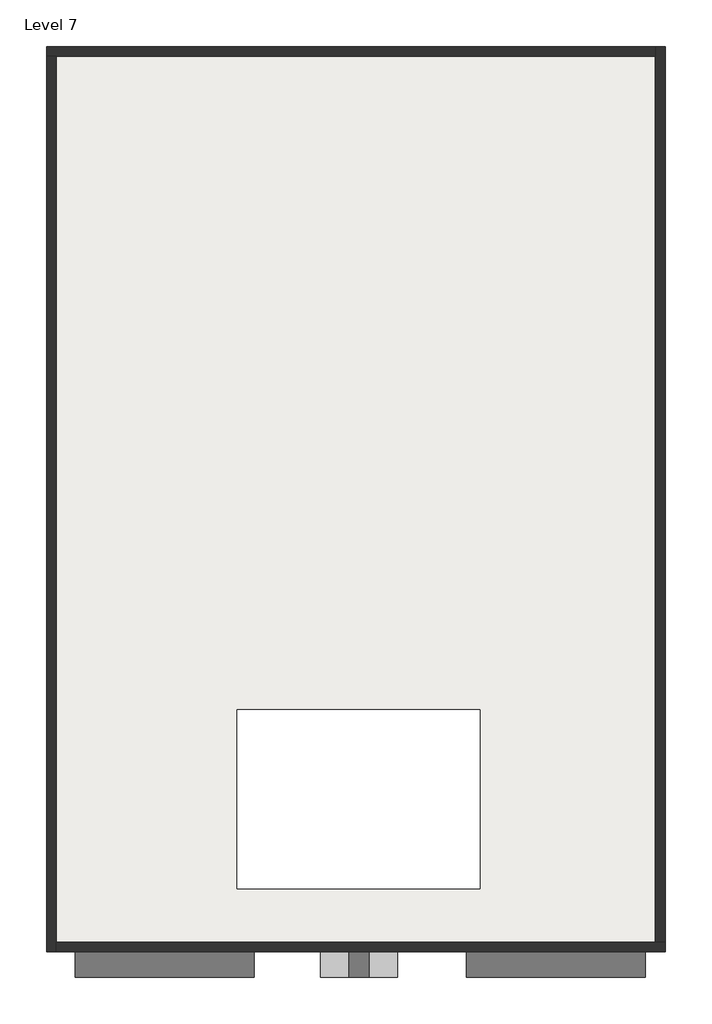
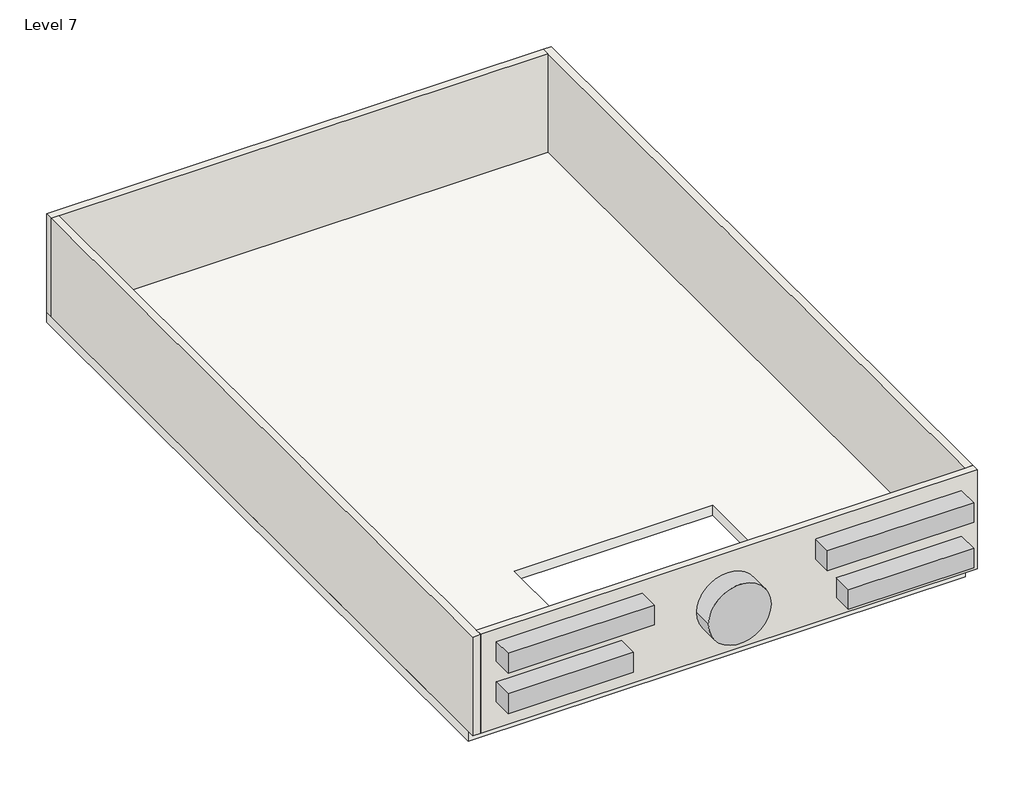
# One storey, incomplete: 4 walls, 1 proxy, 1 roof.
"""IFC4 building model written with IfcOpenShell, lengths in millimetres."""

from ifc_helpers import new_model, si_unit, frame, origin, place, context, project, spatial, polyline, outline, extrude, faceted_brep, transform, mapped, element, save
from components import generic_models_1_generic_models_1_124607eb

model = new_model("IFC4")

# Units and contexts
model_context = context("Model", 3, world=origin())
ifc_project = project(units=[si_unit("LENGTHUNIT", "METRE", prefix="MILLI")], contexts=[model_context])

# Site, building, storey
site = spatial("IfcSite", under=ifc_project)
building = spatial("IfcBuilding", under=site)
storey = spatial("IfcBuildingStorey", under=building, Name="Level 7", Elevation=16002.0)

# Proxy
placement = place(None, origin())
generic_models_1_generic_models_1_shape = generic_models_1_generic_models_1_124607eb(model_context)
element("IfcBuildingElementProxy", 1, Name="Generic Models 1 : Generic Models 1", ObjectType="Generic Models 1 : Generic Models 1", at=placement, inside=storey, context=model_context, shape_type="MappedRepresentation", body=[
    mapped(generic_models_1_generic_models_1_shape, transform((0.0, 0.0, 0.0), x_axis=(1.0, 0.0, 0.0), y_axis=(0.0, 1.0, 0.0), z_axis=(0.0, 0.0, 1.0))),
])

# Roof
element("IfcRoof", 2, ObjectType="Generic - 12\"", at=placement, inside=storey, context=model_context, shape_type="SweptSolid", body=[
    extrude(outline(polyline([(2221.2910386, -5039.0109248), (-5036.7589614, -5039.0109248), (-5036.7589614, 5628.9890752), (2221.2910386, 5628.9890752), (2221.2910386, -5039.0109248)]), holes=[polyline([(131.1896864, -2269.417212), (-2764.4103136, -2269.417212), (-2764.4103136, -4403.017212), (131.1896864, -4403.017212), (131.1896864, -2269.417212)])]), frame((0.0, 0.0, 15849.6), z_axis=(0.0, 0.0, 1.0), x_axis=(1.0, 0.0, 0.0)), (0.0, 0.0, 1.0), 152.4),
])

# Walls
element("IfcWall", 3, ObjectType="4.5\"", at=placement, inside=storey, context=model_context, shape_type="Brep", body=[
    faceted_brep([(-5036.7589614, 5514.6890752, 16002.0), (-4922.4589614, 5514.6890752, 16002.0), (2221.2910386, 5514.6890752, 16002.0), (2221.2910386, 5514.6890752, 17526.0), (-4922.4589614, 5514.6890752, 17526.0), (-5036.7589614, 5514.6890752, 17526.0), (-5036.7589614, 5628.9890752, 16002.0), (-5036.7589614, 5628.9890752, 17526.0), (2221.2910386, 5628.9890752, 17526.0), (2221.2910386, 5628.9890752, 16002.0)], [[[0, 1, 2, 3, 4, 5]], [[6, 7, 8, 9]], [[2, 1, 0, 6, 9]], [[5, 4, 3, 8, 7]], [[0, 5, 7, 6]], [[3, 2, 9, 8]]]),
])
element("IfcWall", 4, ObjectType="4.5\"", at=placement, inside=storey, context=model_context, shape_type="Brep", body=[
    faceted_brep([(-4922.4589614, -5153.3109248, 16002.0), (-4922.4589614, -5039.0109248, 16002.0), (-4922.4589614, 5514.6890752, 16002.0), (-4922.4589614, 5514.6890752, 17526.0), (-4922.4589614, -5039.0109248, 17526.0), (-4922.4589614, -5153.3109248, 17526.0), (-5036.7589614, -5153.3109248, 16002.0), (-5036.7589614, -5153.3109248, 17526.0), (-5036.7589614, 5514.6890752, 17526.0), (-5036.7589614, 5514.6890752, 16002.0)], [[[0, 1, 2, 3, 4, 5]], [[6, 7, 8, 9]], [[2, 1, 0, 6, 9]], [[5, 4, 3, 8, 7]], [[0, 5, 7, 6]], [[3, 2, 9, 8]]]),
])
element("IfcWall", 5, ObjectType="4.5\"", at=placement, inside=storey, context=model_context, shape_type="Brep", body=[
    faceted_brep([(2335.5910386, -5039.0109248, 16002.0), (2221.2910386, -5039.0109248, 16002.0), (-4922.4589614, -5039.0109248, 16002.0), (-4922.4589614, -5039.0109248, 17526.0), (2221.2910386, -5039.0109248, 17526.0), (2335.5910386, -5039.0109248, 17526.0), (2335.5910386, -5153.3109248, 16002.0), (2335.5910386, -5153.3109248, 17526.0), (-4922.4589614, -5153.3109248, 17526.0), (-4922.4589614, -5153.3109248, 16002.0)], [[[0, 1, 2, 3, 4, 5]], [[6, 7, 8, 9]], [[2, 1, 0, 6, 9]], [[5, 4, 3, 8, 7]], [[0, 5, 7, 6]], [[3, 2, 9, 8]]]),
])
element("IfcWall", 6, ObjectType="4.5\"", at=placement, inside=storey, context=model_context, shape_type="Brep", body=[
    faceted_brep([(2221.2910386, 5628.9890752, 16002.0), (2221.2910386, 5514.6890752, 16002.0), (2221.2910386, -5039.0109248, 16002.0), (2221.2910386, -5039.0109248, 17526.0), (2221.2910386, 5514.6890752, 17526.0), (2221.2910386, 5628.9890752, 17526.0), (2335.5910386, 5628.9890752, 16002.0), (2335.5910386, 5628.9890752, 17526.0), (2335.5910386, -5039.0109248, 17526.0), (2335.5910386, -5039.0109248, 16002.0)], [[[0, 1, 2, 3, 4, 5]], [[6, 7, 8, 9]], [[2, 1, 0, 6, 9]], [[5, 4, 3, 8, 7]], [[0, 5, 7, 6]], [[3, 2, 9, 8]]]),
])

save(model, "model.ifc")

# Revit data of these elements
# Type "Generic - 12\""
#   Assembly Code = "B1020"
#   Layers, outside or top first: 0' - 6" no material (function 1)
# Type "4.5\""
#   Assembly Code = "B2010"
#   Layers, outside or top first: 0' - 4 1/2" no material (function 1)
# Element 1 (IfcBuildingElementProxy, "Generic Models 1 : Generic Models 1")
#   Phase Created = New Construction
#   Materials on its faces: "Default Mass Exterior Wall", "Parking Stripe"
# Element 2 (IfcRoof, "Generic - 12\"")
#   built-in parameter 1001705 = 52.5 (stored number, unit not read)
#   built-in parameter 1001701 = -0.5 (stored number, unit not read)
#   built-in parameter 1001710 = 33615
#   Phase Created = New Construction
#   Materials on its faces: "Default Roof", "Door - Frame"
# Elements 3, 4, 5, 6 (IfcWall, "4.5\"")
#   Top Offset = 0' - 0"
#   Base Offset = 0' - 0"
#   Unconnected Height = 5' - 0"
#   wall height = 5' - 0"
#   Phase Created = New Construction
#   Base Constraint = Level 7
#   Materials on its faces: "Default Wall", "Laminate, Ivory, Matte"
# Materials
#   "Default Mass Exterior Wall": class "Generic", colour RGB 133 178 44, transparency 0.2, Cost = 0
#   "Parking Stripe": class "Paint", colour RGB 250 250 91, transparency 0, Cost = 0
#   "Default Roof": colour RGB 88 101 114, transparency 0, Cost = 0
#   "Door - Frame": colour RGB 118 70 51, transparency 0, Cost = 0
#   "Default Wall": colour RGB 128 128 128, transparency 0, Cost = 0
#   "Laminate, Ivory, Matte": class "Plastic", colour RGB 247 247 239, transparency 0, Description = "Plastic Laminate - Ivory, Matte", Cost = 0
